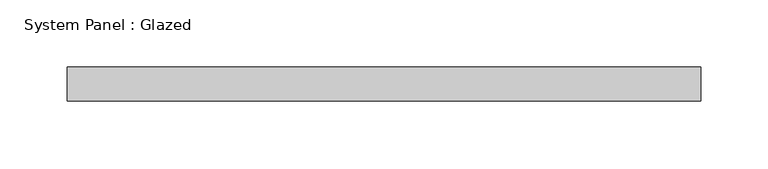
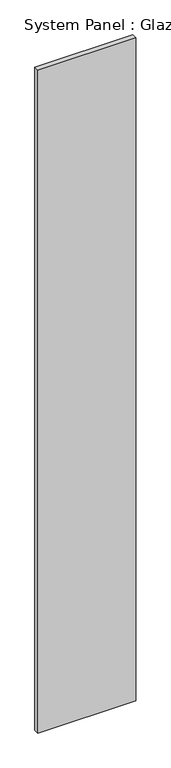
"""IFC4 building model written with IfcOpenShell, lengths in millimetres: plate geometry, System Panel : Glazed."""

from ifc_helpers import new_model, si_unit, origin, origin_with_axes, place, context, project, spatial, polyline, outline, extrude, source, transform, mapped, element, save


def system_panel_glazed_aeaff5c2(model_context):
    return source(origin(), model_context, "Body", "SweptSolid", [
        extrude(outline(polyline([(236.225, 19.05), (-236.225, 19.05), (-236.225, 44.45), (236.225, 44.45), (236.225, 19.05)])), origin_with_axes(), (0.0, 0.0, 1.0), 3379.9820397),
    ])


if __name__ == "__main__":
    model = new_model("IFC4")
    model_context = context("Model", 3, world=origin())
    ifc_project = project(units=[si_unit("LENGTHUNIT", "METRE", prefix="MILLI")], contexts=[model_context])
    site = spatial("IfcSite", under=ifc_project)
    building = spatial("IfcBuilding", under=site)
    placement = place(None, origin())
    system_panel_glazed_shape = system_panel_glazed_aeaff5c2(model_context)
    element("IfcPlate", 1, ObjectType="System Panel : Glazed", at=placement, inside=building, context=model_context, shape_type="MappedRepresentation", body=[
        mapped(system_panel_glazed_shape, transform((0.0, 0.0, 0.0), x_axis=(1.0, 0.0, 0.0), y_axis=(0.0, 1.0, 0.0), z_axis=(0.0, 0.0, 1.0))),
    ])
    save(model, "model.ifc")

# Revit data of these elements
# Type "System Panel : Glazed"
#   Construction Type Id = "GSP4R"
#   Analytic Construction = "1/8 in Pilkington single glazing"
#   Visual Light Transmittance = 0.9
#   Solar Heat Gain Coefficient = 0.86
#   Heat Transfer Coefficient (U) = 1.18115 BTU/(h·ft²·°F)
#   Define Thermal Properties by = 1
# Element 1 (IfcPlate, "System Panel : Glazed")
#   Materials on its faces: "Glass"
# Materials
#   "Glass": class "Glass", colour RGB 0 128 192, transparency 0.75, Description = "Soda Lime Glass", Cost = 0
